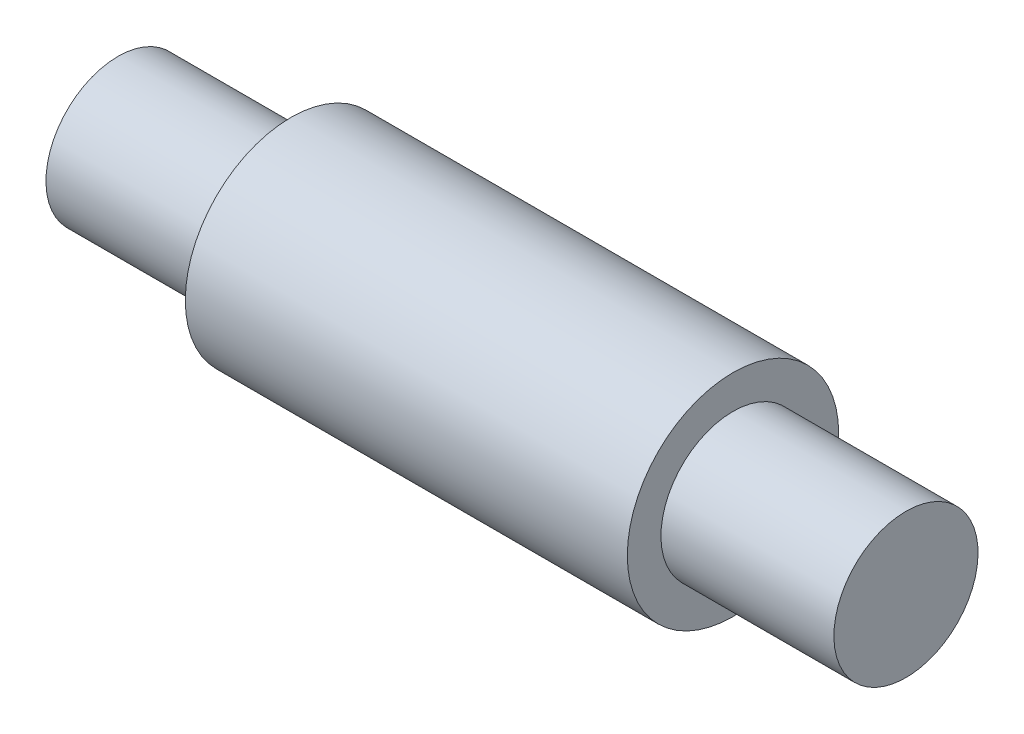
ISO-10303-21;
HEADER;
FILE_DESCRIPTION(('STEP AP214'),'2;1');
FILE_NAME('part.step','',(''),(''),'','','');
FILE_SCHEMA(('AUTOMOTIVE_DESIGN { 1 0 10303 214 1 1 1 1 }'));
ENDSEC;
DATA;
#1=APPLICATION_CONTEXT('core data for automotive mechanical design processes');
#2=APPLICATION_PROTOCOL_DEFINITION('international standard','automotive_design',2000,#1);
#3=PRODUCT_CONTEXT('',#1,'mechanical');
#4=PRODUCT('Part','Part','',(#3));
#5=PRODUCT_RELATED_PRODUCT_CATEGORY('part','',(#4));
#6=PRODUCT_DEFINITION_FORMATION('','',#4);
#7=PRODUCT_DEFINITION_CONTEXT('part definition',#1,'design');
#8=PRODUCT_DEFINITION('design','',#6,#7);
#9=PRODUCT_DEFINITION_SHAPE('','',#8);
#10=(LENGTH_UNIT() NAMED_UNIT(*) SI_UNIT(.MILLI.,.METRE.));
#11=(NAMED_UNIT(*) PLANE_ANGLE_UNIT() SI_UNIT($,.RADIAN.));
#12=(NAMED_UNIT(*) SI_UNIT($,.STERADIAN.) SOLID_ANGLE_UNIT());
#13=UNCERTAINTY_MEASURE_WITH_UNIT(LENGTH_MEASURE(1.E-05),#10,'distance_accuracy_value','');
#14=(GEOMETRIC_REPRESENTATION_CONTEXT(3) GLOBAL_UNCERTAINTY_ASSIGNED_CONTEXT((#13)) GLOBAL_UNIT_ASSIGNED_CONTEXT((#10,
#11,#12)) REPRESENTATION_CONTEXT('',''));
#15=CARTESIAN_POINT('',(0.,0.,0.));
#16=DIRECTION('',(0.,0.,1.));
#17=DIRECTION('',(1.,0.,0.));
#18=AXIS2_PLACEMENT_3D('',#15,#16,#17);
#19=CARTESIAN_POINT('',(-82.,0.,0.));
#20=DIRECTION('',(-1.,0.,0.));
#21=DIRECTION('',(0.,-1.,0.));
#22=AXIS2_PLACEMENT_3D('',#19,#20,#21);
#23=PLANE('',#22);
#24=CARTESIAN_POINT('',(-82.,0.,0.));
#25=DIRECTION('',(1.,0.,0.));
#26=DIRECTION('',(0.,1.,0.));
#27=AXIS2_PLACEMENT_3D('',#24,#25,#26);
#28=CIRCLE('',#27,7.5);
#29=CARTESIAN_POINT('',(-82.,7.49999999999999,0.));
#30=VERTEX_POINT('',#29);
#31=EDGE_CURVE('E10',#30,#30,#28,.T.);
#32=ORIENTED_EDGE('',*,*,#31,.F.);
#33=EDGE_LOOP('',(#32));
#34=FACE_BOUND('',#33,.T.);
#35=ADVANCED_FACE('F50',(#34),#23,.T.);
#36=CARTESIAN_POINT('',(0.,0.,0.));
#37=DIRECTION('',(1.,0.,0.));
#38=DIRECTION('',(0.,1.,0.));
#39=AXIS2_PLACEMENT_3D('',#36,#37,#38);
#40=CYLINDRICAL_SURFACE('',#39,7.5);
#41=ORIENTED_EDGE('',*,*,#31,.T.);
#42=EDGE_LOOP('',(#41));
#43=FACE_BOUND('',#42,.T.);
#44=CARTESIAN_POINT('',(-64.,0.,0.));
#45=DIRECTION('',(1.,0.,0.));
#46=DIRECTION('',(0.,1.,0.));
#47=AXIS2_PLACEMENT_3D('',#44,#45,#46);
#48=CIRCLE('',#47,7.5);
#49=CARTESIAN_POINT('',(-64.,7.49999999999999,0.));
#50=VERTEX_POINT('',#49);
#51=EDGE_CURVE('E52',#50,#50,#48,.T.);
#52=ORIENTED_EDGE('',*,*,#51,.F.);
#53=EDGE_LOOP('',(#52));
#54=FACE_BOUND('',#53,.T.);
#55=ADVANCED_FACE('F90',(#43,#54),#40,.T.);
#56=CARTESIAN_POINT('',(-64.,7.49999999999999,0.));
#57=DIRECTION('',(-1.,0.,0.));
#58=DIRECTION('',(0.,-1.,0.));
#59=AXIS2_PLACEMENT_3D('',#56,#57,#58);
#60=PLANE('',#59);
#61=ORIENTED_EDGE('',*,*,#51,.T.);
#62=EDGE_LOOP('',(#61));
#63=FACE_BOUND('',#62,.T.);
#64=CARTESIAN_POINT('',(-64.,0.,0.));
#65=DIRECTION('',(1.,0.,0.));
#66=DIRECTION('',(0.,1.,0.));
#67=AXIS2_PLACEMENT_3D('',#64,#65,#66);
#68=CIRCLE('',#67,11.);
#69=CARTESIAN_POINT('',(-64.,11.,0.));
#70=VERTEX_POINT('',#69);
#71=EDGE_CURVE('E60',#70,#70,#68,.T.);
#72=ORIENTED_EDGE('',*,*,#71,.F.);
#73=EDGE_LOOP('',(#72));
#74=FACE_BOUND('',#73,.T.);
#75=ADVANCED_FACE('F92',(#63,#74),#60,.T.);
#76=CARTESIAN_POINT('',(0.,0.,0.));
#77=DIRECTION('',(1.,0.,0.));
#78=DIRECTION('',(0.,1.,0.));
#79=AXIS2_PLACEMENT_3D('',#76,#77,#78);
#80=CYLINDRICAL_SURFACE('',#79,11.);
#81=ORIENTED_EDGE('',*,*,#71,.T.);
#82=EDGE_LOOP('',(#81));
#83=FACE_BOUND('',#82,.T.);
#84=CARTESIAN_POINT('',(-18.,0.,0.));
#85=DIRECTION('',(1.,0.,0.));
#86=DIRECTION('',(0.,1.,0.));
#87=AXIS2_PLACEMENT_3D('',#84,#85,#86);
#88=CIRCLE('',#87,11.);
#89=CARTESIAN_POINT('',(-18.,11.,0.));
#90=VERTEX_POINT('',#89);
#91=EDGE_CURVE('E63',#90,#90,#88,.T.);
#92=ORIENTED_EDGE('',*,*,#91,.F.);
#93=EDGE_LOOP('',(#92));
#94=FACE_BOUND('',#93,.T.);
#95=ADVANCED_FACE('F82',(#83,#94),#80,.T.);
#96=CARTESIAN_POINT('',(-18.,11.,0.));
#97=DIRECTION('',(1.,0.,0.));
#98=DIRECTION('',(0.,1.,0.));
#99=AXIS2_PLACEMENT_3D('',#96,#97,#98);
#100=PLANE('',#99);
#101=ORIENTED_EDGE('',*,*,#91,.T.);
#102=EDGE_LOOP('',(#101));
#103=FACE_BOUND('',#102,.T.);
#104=CARTESIAN_POINT('',(-18.,0.,0.));
#105=DIRECTION('',(1.,0.,0.));
#106=DIRECTION('',(0.,1.,0.));
#107=AXIS2_PLACEMENT_3D('',#104,#105,#106);
#108=CIRCLE('',#107,7.5);
#109=CARTESIAN_POINT('',(-18.,7.5,0.));
#110=VERTEX_POINT('',#109);
#111=EDGE_CURVE('E69',#110,#110,#108,.T.);
#112=ORIENTED_EDGE('',*,*,#111,.F.);
#113=EDGE_LOOP('',(#112));
#114=FACE_BOUND('',#113,.T.);
#115=ADVANCED_FACE('F79',(#103,#114),#100,.T.);
#116=CARTESIAN_POINT('',(0.,0.,0.));
#117=DIRECTION('',(1.,0.,0.));
#118=DIRECTION('',(0.,1.,0.));
#119=AXIS2_PLACEMENT_3D('',#116,#117,#118);
#120=CYLINDRICAL_SURFACE('',#119,7.5);
#121=ORIENTED_EDGE('',*,*,#111,.T.);
#122=EDGE_LOOP('',(#121));
#123=FACE_BOUND('',#122,.T.);
#124=CARTESIAN_POINT('',(0.,0.,0.));
#125=DIRECTION('',(1.,0.,0.));
#126=DIRECTION('',(0.,1.,0.));
#127=AXIS2_PLACEMENT_3D('',#124,#125,#126);
#128=CIRCLE('',#127,7.5);
#129=CARTESIAN_POINT('',(0.,7.5,0.));
#130=VERTEX_POINT('',#129);
#131=EDGE_CURVE('E68',#130,#130,#128,.T.);
#132=ORIENTED_EDGE('',*,*,#131,.F.);
#133=EDGE_LOOP('',(#132));
#134=FACE_BOUND('',#133,.T.);
#135=ADVANCED_FACE('F73',(#123,#134),#120,.T.);
#136=CARTESIAN_POINT('',(0.,7.5,0.));
#137=DIRECTION('',(1.,0.,0.));
#138=DIRECTION('',(0.,1.,0.));
#139=AXIS2_PLACEMENT_3D('',#136,#137,#138);
#140=PLANE('',#139);
#141=ORIENTED_EDGE('',*,*,#131,.T.);
#142=EDGE_LOOP('',(#141));
#143=FACE_BOUND('',#142,.T.);
#144=ADVANCED_FACE('F71',(#143),#140,.T.);
#145=CLOSED_SHELL('',(#35,#55,#75,#95,#115,#135,#144));
#146=MANIFOLD_SOLID_BREP('B2',#145);
#147=ADVANCED_BREP_SHAPE_REPRESENTATION('',(#18,#146),#14);
#148=SHAPE_DEFINITION_REPRESENTATION(#9,#147);
ENDSEC;
END-ISO-10303-21;
